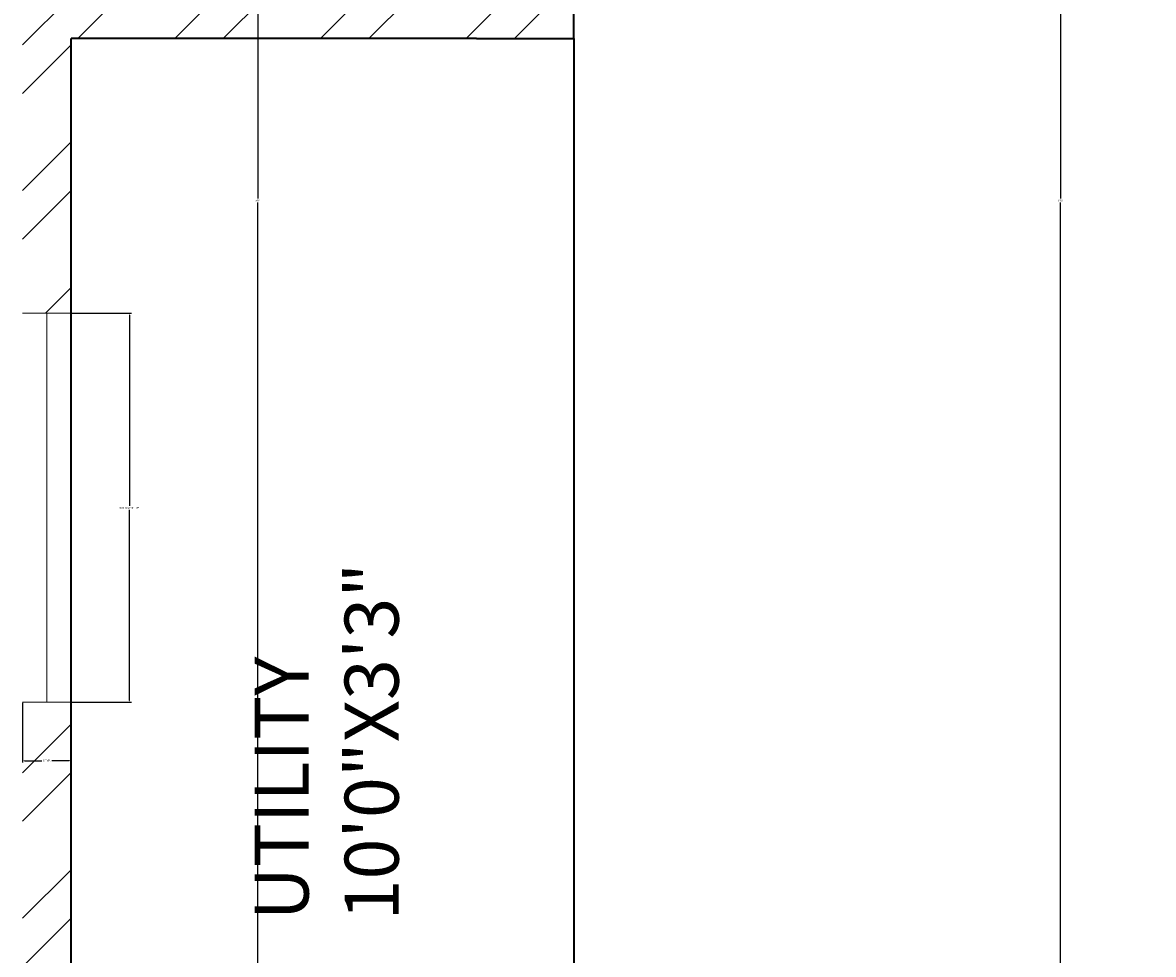
# Model space of a CAD drawing. Units: inches. Extents: x 2120 to 4013, y 1390 to 3019.
# Tile 26 of 59: x 2959 to 3063, y 1878 to 1964. Entities that reach past the tile are written whole.
import ezdxf

# ---------------------------------------------------------------- set-up
doc = ezdxf.new("R2010")
doc.units = ezdxf.units.IN
for name, color, linetype, lineweight in [('A-ANNO-DIMS', 2, 'Continuous', 18), ('A-AREA-IDEN', 7, 'Continuous', 18), ('A-GLAZ', 4, 'Continuous', 18), ('A-WALL', 7, 'Continuous', 35), ('A-WALL-PATT', 252, 'Continuous', 13)]:
    doc.layers.add(name, color=color, linetype=linetype, lineweight=lineweight)
doc.styles.get("Standard").update_dxf_attribs({"font": 'arial.ttf'})
doc.dimstyles.get("Standard").update_dxf_attribs({"dimtxt": 0.18, "dimasz": 0.18, "dimexe": 0.18, "dimexo": 0.0625, "dimgap": 0.09, "dimtad": 0, "dimtih": 1, "dimtoh": 1, "dimdec": 4, "dimzin": 0, "dimdsep": 46, "dimtxsty": 'Standard', "dimcen": 0.09, "dimadec": 0, "dimazin": 0, "dimtfac": 1, "dimtdec": 4, "dimtofl": 0, "dimtmove": 0, "dimatfit": 3, "dimfxl": 1, "dimtolj": 1, "dimtzin": 0, "dimarcsym": 0})

# ---------------------------------------------------------------- blocks, each defined once
blk = doc.blocks.new('WIN-PLAN-36IN-02')
for p, q in [((2.25, 36), (0, 36)), ((0, 36), (4.5, 36)), ((2.25, 0), (2.25, 36)), ((0, 0), (4.5, 0)), ((4.5, 0), (2.25, 0))]:
    blk.add_line(p, q)
blk = doc.blocks.new('*D179')
at = {"layer": 'A-ANNO-DIMS', "color": 0, "lineweight": -2, "transparency": 16777216}
for p, q in [((2963.3, 1937.09), (2968.81, 1937.09)), ((2968.63, 1936.91), (2968.63, 1919.28)), ((2968.63, 1901.27), (2968.63, 1918.91)), ((2963.3, 1901.09), (2968.81, 1901.09))]:
    blk.add_line(p, q, dxfattribs=at)
at = {"layer": 'A-ANNO-DIMS', "color": 0, "transparency": 16777216}
for points in [[(2968.6, 1936.91), (2968.66, 1936.91), (2968.63, 1937.09)], [(2968.6, 1901.27), (2968.66, 1901.27), (2968.63, 1901.09)]]:
    blk.add_solid(points, dxfattribs=at)
at = {"layer": 'Defpoints', "color": 0, "transparency": 16777216}
for p in [(2963.23, 1937.09), (2968.63, 1937.09), (2963.23, 1901.09)]:
    blk.add_point(p, dxfattribs=at)
at = {"layer": 'A-ANNO-DIMS', "color": 0, "transparency": 16777216, "insert": (2968.63, 1919.09), "char_height": 0.18, "attachment_point": 5}
blk.add_mtext('\\A1;WINDOW 36 TYP.', dxfattribs=at)
blk = doc.blocks.new('*D180')
at = {"layer": 'A-ANNO-DIMS', "color": 0, "lineweight": -2, "transparency": 16777216}
for p, q in [((2958.73, 1901.03), (2958.73, 1895.51)), ((2963.23, 1901.03), (2963.23, 1895.51)), ((2958.91, 1895.69), (2960.52, 1895.69)), ((2963.05, 1895.69), (2961.44, 1895.69))]:
    blk.add_line(p, q, dxfattribs=at)
at = {"layer": 'A-ANNO-DIMS', "color": 0, "transparency": 16777216}
for points in [[(2958.91, 1895.72), (2958.91, 1895.66), (2958.73, 1895.69)], [(2963.05, 1895.72), (2963.05, 1895.66), (2963.23, 1895.69)]]:
    blk.add_solid(points, dxfattribs=at)
at = {"layer": 'Defpoints', "color": 0, "transparency": 16777216}
for p in [(2958.73, 1901.09), (2963.23, 1901.09), (2963.23, 1895.69)]:
    blk.add_point(p, dxfattribs=at)
at = {"layer": 'A-ANNO-DIMS', "color": 0, "transparency": 16777216, "insert": (2960.98, 1895.69), "char_height": 0.18, "attachment_point": 5}
blk.add_mtext('\\A1;5 TYP.', dxfattribs=at)
blk = doc.blocks.new('*D212')
at = {"layer": 'A-ANNO-DIMS', "color": 0, "lineweight": -2, "transparency": 16777216}
for p, q in [((3009.8, 2352.53), (3054.91, 2352.53)), ((3054.73, 2352.35), (3054.73, 1947.71)), ((3054.73, 1542.71), (3054.73, 1947.35)), ((3009.8, 1542.53), (3054.91, 1542.53))]:
    blk.add_line(p, q, dxfattribs=at)
at = {"layer": 'A-ANNO-DIMS', "color": 0, "transparency": 16777216}
for points in [[(3054.7, 2352.35), (3054.76, 2352.35), (3054.73, 2352.53)], [(3054.7, 1542.71), (3054.76, 1542.71), (3054.73, 1542.53)]]:
    blk.add_solid(points, dxfattribs=at)
at = {"layer": 'Defpoints', "color": 0, "transparency": 16777216}
for p in [(3009.73, 2352.53), (3009.73, 1542.53), (3054.73, 1542.53)]:
    blk.add_point(p, dxfattribs=at)
at = {"layer": 'A-ANNO-DIMS', "color": 0, "transparency": 16777216, "insert": (3054.73, 1947.53), "char_height": 0.18, "attachment_point": 5}
blk.add_mtext('\\A1;810', dxfattribs=at)
blk = doc.blocks.new('*D217')
at = {"layer": 'A-ANNO-DIMS', "color": 0, "lineweight": -2, "transparency": 16777216}
for p, q in [((3071.67, 2352.53), (2980.31, 2352.53)), ((2980.49, 2352.35), (2980.49, 1947.71)), ((2980.49, 1542.71), (2980.49, 1947.35)), ((3305.67, 1542.53), (2980.31, 1542.53))]:
    blk.add_line(p, q, dxfattribs=at)
at = {"layer": 'A-ANNO-DIMS', "color": 0, "transparency": 16777216}
for points in [[(2980.46, 2352.35), (2980.52, 2352.35), (2980.49, 2352.53)], [(2980.46, 1542.71), (2980.52, 1542.71), (2980.49, 1542.53)]]:
    blk.add_solid(points, dxfattribs=at)
at = {"layer": 'Defpoints', "color": 0, "transparency": 16777216}
for p in [(2980.49, 2352.53), (3071.73, 2352.53), (3305.73, 1542.53)]:
    blk.add_point(p, dxfattribs=at)
at = {"layer": 'A-ANNO-DIMS', "color": 0, "transparency": 16777216, "insert": (2980.49, 1947.53), "char_height": 0.18, "attachment_point": 5}
blk.add_mtext('\\A1;810', dxfattribs=at)

msp = doc.modelspace()

# ---------------------------------------------------------------- hatches: boundary and pattern name
at = {"layer": 'A-WALL-PATT'}
h = msp.add_hatch(dxfattribs=at)
h.set_pattern_fill('ANSI32', color=256)
h.paths.add_polyline_path([(2271.7331, 2343.531), (2283.3788, 2343.531), (2283.3788, 2348.031), (2283.3788, 2352.5306), (2262.7331, 2352.5306), (2262.7331, 2182.638), (2267.2331, 2182.638), (2271.7331, 2182.638), (2271.7331, 2219.031), (2391.7331, 2219.031), (2391.7331, 2214.189), (2393.9831, 2214.189), (2396.2331, 2214.189), (2396.2331, 2219.031), (2420.2331, 2219.031), (2420.2331, 2225.7535), (2417.2197, 2225.7535), (2415.7331, 2225.7535), (2415.7331, 2223.5306), (2271.7331, 2223.5306)])
h.paths.add_polyline_path([(2380.0942, 2352.5306), (2343.3788, 2352.5306), (2343.3788, 2343.531), (2363.2331, 2343.531), (2363.2331, 2288.8489), (2365.4831, 2288.8489), (2367.7331, 2288.8489), (2367.7331, 2343.531), (2380.0942, 2343.531)], flags=17)
h.paths.add_polyline_path([(2432.4339, 2352.5306), (2404.0943, 2352.5306), (2404.0943, 2343.531), (2415.7331, 2343.531), (2415.7331, 2264.0306), (2367.7331, 2264.0306), (2367.7331, 2266.4872), (2363.2331, 2266.4872), (2363.2331, 2259.531), (2367.7331, 2259.531), (2415.7331, 2259.531), (2415.7331, 2255.0658), (2420.2331, 2255.0658), (2420.2331, 2259.531), (2424.5717, 2259.531), (2424.5717, 2261.781), (2424.5717, 2264.0306), (2420.2331, 2264.0306), (2420.2331, 2343.531), (2432.4339, 2343.531)])
h.paths.add_polyline_path([(2508.9115, 2352.5306), (2456.4339, 2352.5306), (2456.4339, 2343.531), (2468.2331, 2343.531), (2468.2331, 2264.0306), (2448.0487, 2264.0306), (2448.0487, 2259.531), (2468.2331, 2259.531), (2468.2331, 2255.5496), (2472.7331, 2255.5496), (2472.7331, 2343.531), (2508.9115, 2343.531)])
h.paths.add_polyline_path([(2637.7331, 2352.5306), (2544.9116, 2352.5306), (2544.9116, 2343.531), (2589.7331, 2343.531), (2633.2331, 2343.531), (2637.7331, 2343.531)])
h.paths.add_polyline_path([(2594.2331, 2343.5306), (2589.7331, 2343.5306), (2589.7331, 2259.5306), (2589.7331, 2252.4915), (2591.9831, 2252.4915), (2594.2331, 2252.4915)])
h.paths.add_polyline_path([(2637.7331, 2223.5306), (2594.2331, 2223.5306), (2594.2331, 2230.1988), (2591.9831, 2230.1988), (2589.7331, 2230.1988), (2589.7331, 2223.5306), (2472.7331, 2223.5306), (2468.2331, 2223.5306), (2468.2331, 2219.031), (2628.7331, 2219.031), (2628.7331, 2138.031), (2637.7331, 2138.031)])
h.paths.add_polyline_path([(3822.6535, 2458.4402), (3874.9468, 2458.4402), (3874.9468, 2476.9866), (3822.6535, 2476.9866)], flags=9)
h.paths.add_polyline_path([(3834.6921, 2781.8174), (3935.9206, 2781.8174), (3935.9206, 2800.3638), (3834.6921, 2800.3638)], flags=9)
h.paths.add_polyline_path([(3832.2843, 2837.9683), (3884.5776, 2837.9683), (3884.5776, 2856.5146), (3832.2843, 2856.5146)], flags=9)
h.paths.add_polyline_path([(3830.9388, 2861.4782), (3956.8958, 2861.4782), (3956.8958, 2880.0245), (3830.9388, 2880.0245)], flags=9)
h.paths.add_polyline_path([(3870.6966, 2352.5752), (3887.9272, 2352.5752), (3887.9272, 2377.3037), (3870.6966, 2377.3037)], flags=9)
h.paths.add_polyline_path([(3289.2701, 2413.161), (3435.2223, 2413.161), (3435.2223, 2450.2538), (3289.2701, 2450.2538)], flags=9)
h.paths.add_polyline_path([(2487.6944, 2414.3601), (2637.8335, 2414.3601), (2637.8335, 2451.4528), (2487.6944, 2451.4528)], flags=9)
h.paths.add_polyline_path([(2567.3724, 1457.9199), (2815.296, 1457.9199), (2815.296, 1495.0127), (2567.3724, 1495.0127)], flags=9)
h.paths.add_polyline_path([(2655.3825, 2093.2363), (2685.9555, 2093.2363), (2685.9555, 2111.8937), (2655.3825, 2111.8937)], flags=9)
h.paths.add_polyline_path([(2543.9218, 1550.6671), (2587.8406, 1550.6671), (2587.8406, 1569.3244), (2543.9218, 1569.3244)], flags=9)
h.paths.add_polyline_path([(2905.1384, 1543.8113), (2949.0572, 1543.8113), (2949.0572, 1562.4686), (2905.1384, 1562.4686)], flags=9)
h.paths.add_polyline_path([(2736.4118, 1702.4736), (2784.2153, 1702.4736), (2784.2153, 1721.1309), (2736.4118, 1721.1309)], flags=9)
h.paths.add_polyline_path([(2912.8666, 1710.4168), (2951.707, 1710.4168), (2951.707, 1729.0741), (2912.8666, 1729.0741)], flags=9)
h.paths.add_polyline_path([(2923.5785, 1763.5038), (2959.7279, 1763.5038), (2959.7279, 1782.1611), (2923.5785, 1782.1611)], flags=9)
h.paths.add_polyline_path([(2925.2114, 1809.6137), (2967.1861, 1809.6137), (2967.1861, 1828.271), (2925.2114, 1828.271)], flags=9)
h.paths.add_polyline_path([(2996.2711, 1878.9003), (2996.2711, 1913.109), (2977.6138, 1913.109), (2977.6138, 1878.9003)], flags=9)
h.paths.add_polyline_path([(2883.0859, 1895.7192), (2927.1855, 1895.7192), (2927.1855, 1914.3766), (2883.0859, 1914.3766)], flags=9)
h.paths.add_polyline_path([(2787.3924, 1810.8013), (2841.0213, 1810.8013), (2841.0213, 1829.4587), (2787.3924, 1829.4587)], flags=9)
h.paths.add_polyline_path([(2775.6399, 2101.7395), (2829.2689, 2101.7395), (2829.2689, 2120.3968), (2775.6399, 2120.3968)], flags=9)
h.paths.add_polyline_path([(2913.0263, 2075.817), (2951.8667, 2075.817), (2951.8667, 2094.4744), (2913.0263, 2094.4744)], flags=9)
h.paths.add_polyline_path([(2929.966, 2133.3669), (2966.1154, 2133.3669), (2966.1154, 2152.0243), (2929.966, 2152.0243)], flags=9)
h.paths.add_polyline_path([(2932.7502, 2182.6088), (2968.8996, 2182.6088), (2968.8996, 2201.2662), (2932.7502, 2201.2662)], flags=9)
h.paths.add_polyline_path([(2996.0681, 2266.3173), (2996.0681, 2300.5261), (2977.4108, 2300.5261), (2977.4108, 2266.3173)], flags=9)
h.paths.add_polyline_path([(2885.1039, 2279.2186), (2929.2035, 2279.2186), (2929.2035, 2297.8759), (2885.1039, 2297.8759)], flags=9)
h.paths.add_polyline_path([(2735.7042, 2218.3197), (2783.5078, 2218.3197), (2783.5078, 2236.9771), (2735.7042, 2236.9771)], flags=9)
h.paths.add_polyline_path([(2635.6049, 2044.0085), (2648.9678, 2044.0085), (2648.9678, 2054.312), (2635.6049, 2054.312)], flags=9)
h.paths.add_polyline_path([(2714.0148, 1923.0473), (2727.3777, 1923.0473), (2727.3777, 1933.3508), (2714.0148, 1933.3508)], flags=9)
h.paths.add_polyline_path([(2709.0345, 1988.1628), (2722.3974, 1988.1628), (2722.3974, 1998.4663), (2709.0345, 1998.4663)], flags=9)
h.paths.add_polyline_path([(2592.8935, 1962.1763), (2606.2564, 1962.1763), (2606.2564, 1972.4799), (2592.8935, 1972.4799)], flags=9)
h.paths.add_polyline_path([(2618.3996, 1985.9724), (2644.1942, 1985.9724), (2644.1942, 1996.2759), (2618.3996, 1996.2759)], flags=9)
h.paths.add_polyline_path([(2601.279, 1920.5869), (2614.6419, 1920.5869), (2614.6419, 1930.8904), (2601.279, 1930.8904)], flags=9)
h.paths.add_polyline_path([(2692.3278, 1932.7645), (2704.5311, 1932.7645), (2704.5311, 1943.0681), (2692.3278, 1943.0681)], flags=9)
h.paths.add_polyline_path([(2311.122, 1672.7318), (2355.0408, 1672.7318), (2355.0408, 1691.3892), (2311.122, 1691.3892)], flags=9)
h.paths.add_polyline_path([(2456.2551, 1632.3198), (2492.4796, 1632.3198), (2492.4796, 1650.9772), (2456.2551, 1650.9772)], flags=9)
h.paths.add_polyline_path([(2401.0766, 1631.4793), (2437.301, 1631.4793), (2437.301, 1650.1367), (2401.0766, 1650.1367)], flags=9)
h.paths.add_polyline_path([(2546.7054, 1700.9235), (2594.509, 1700.9235), (2594.509, 1719.5809), (2546.7054, 1719.5809)], flags=9)
h.paths.add_polyline_path([(2445.4866, 1766.9937), (2497.5261, 1766.9937), (2497.5261, 1785.651), (2445.4866, 1785.651)], flags=9)
h.paths.add_polyline_path([(2287.9992, 1739.7675), (2326.8396, 1739.7675), (2326.8396, 1758.4248), (2287.9992, 1758.4248)], flags=9)
h.paths.add_polyline_path([(2458.5279, 1924.7607), (2510.5675, 1924.7607), (2510.5675, 1943.4181), (2458.5279, 1943.4181)], flags=9)
h.paths.add_polyline_path([(2309.2811, 1902.7642), (2345.4305, 1902.7642), (2345.4305, 1921.4215), (2309.2811, 1921.4215)], flags=9)
h.paths.add_polyline_path([(2490.7554, 2018.9392), (2530.7896, 2018.9392), (2530.7896, 2037.5965), (2490.7554, 2037.5965)], flags=9)
h.paths.add_polyline_path([(2402.143, 2024.7393), (2438.5414, 2024.7393), (2438.5414, 2043.3966), (2402.143, 2043.3966)], flags=9)
h.paths.add_polyline_path([(2287.856, 1931.7926), (2326.6964, 1931.7926), (2326.6964, 1950.4499), (2287.856, 1950.4499)], flags=9)
h.paths.add_polyline_path([(2281.7979, 2193.5771), (2320.6383, 2193.5771), (2320.6383, 2212.2344), (2281.7979, 2212.2344)], flags=25)
h.paths.add_polyline_path([(2484.0754, 2093.892), (2536.115, 2093.892), (2536.115, 2112.5494), (2484.0754, 2112.5494)], flags=9)
h.paths.add_polyline_path([(2624.7948, 2281.8639), (2624.7948, 2311.4137), (2606.1375, 2311.4137), (2606.1375, 2281.8639)], flags=9)
h.paths.add_polyline_path([(2507.5036, 2290.3639), (2541.934, 2290.3639), (2541.934, 2309.0212), (2507.5036, 2309.0212)], flags=9)
h.paths.add_polyline_path([(2423.1076, 2285.2202), (2459.332, 2285.2202), (2459.332, 2303.8776), (2423.1076, 2303.8776)], flags=9)
h.paths.add_polyline_path([(2374.5467, 2289.6272), (2410.7711, 2289.6272), (2410.7711, 2308.2846), (2374.5467, 2308.2846)], flags=25)
h.paths.add_polyline_path([(2277.4907, 2227.5651), (2316.3311, 2227.5651), (2316.3311, 2246.2224), (2277.4907, 2246.2224)], flags=25)
h.paths.add_polyline_path([(2655.3825, 2093.2367), (2685.9555, 2093.2367), (2685.9555, 2111.894), (2655.3825, 2111.894)], flags=9)
h.paths.add_polyline_path([(2543.9217, 1550.6674), (2587.8406, 1550.6674), (2587.8406, 1569.3247), (2543.9217, 1569.3247)], flags=9)
h.paths.add_polyline_path([(2905.1384, 1543.8116), (2949.0572, 1543.8116), (2949.0572, 1562.4689), (2905.1384, 1562.4689)], flags=9)
h.paths.add_polyline_path([(2736.4118, 1702.4739), (2784.2153, 1702.4739), (2784.2153, 1721.1312), (2736.4118, 1721.1312)], flags=9)
h.paths.add_polyline_path([(2912.8666, 1710.4171), (2951.707, 1710.4171), (2951.707, 1729.0744), (2912.8666, 1729.0744)], flags=9)
h.paths.add_polyline_path([(2923.5785, 1763.5041), (2959.7279, 1763.5041), (2959.7279, 1782.1614), (2923.5785, 1782.1614)], flags=9)
h.paths.add_polyline_path([(2925.2114, 1809.614), (2967.1861, 1809.614), (2967.1861, 1828.2713), (2925.2114, 1828.2713)], flags=9)
h.paths.add_polyline_path([(2996.2711, 1878.9006), (2996.2711, 1913.1094), (2977.6137, 1913.1094), (2977.6137, 1878.9006)], flags=9)
h.paths.add_polyline_path([(2883.0859, 1895.7195), (2927.1855, 1895.7195), (2927.1855, 1914.3769), (2883.0859, 1914.3769)], flags=9)
h.paths.add_polyline_path([(2787.3924, 1810.8016), (2841.0213, 1810.8016), (2841.0213, 1829.459), (2787.3924, 1829.459)], flags=9)
h.paths.add_polyline_path([(2775.6399, 2101.7398), (2829.2688, 2101.7398), (2829.2688, 2120.3971), (2775.6399, 2120.3971)], flags=9)
h.paths.add_polyline_path([(2913.0263, 2075.8173), (2951.8667, 2075.8173), (2951.8667, 2094.4747), (2913.0263, 2094.4747)], flags=9)
h.paths.add_polyline_path([(2929.966, 2133.3672), (2966.1154, 2133.3672), (2966.1154, 2152.0246), (2929.966, 2152.0246)], flags=9)
h.paths.add_polyline_path([(2932.7502, 2182.6091), (2968.8996, 2182.6091), (2968.8996, 2201.2665), (2932.7502, 2201.2665)], flags=9)
h.paths.add_polyline_path([(2996.0681, 2266.3176), (2996.0681, 2300.5264), (2977.4108, 2300.5264), (2977.4108, 2266.3176)], flags=9)
h.paths.add_polyline_path([(2885.1039, 2279.2189), (2929.2035, 2279.2189), (2929.2035, 2297.8762), (2885.1039, 2297.8762)], flags=9)
h.paths.add_polyline_path([(2735.7042, 2218.32), (2783.5078, 2218.32), (2783.5078, 2236.9774), (2735.7042, 2236.9774)], flags=9)
h.paths.add_polyline_path([(2635.6048, 2044.0088), (2648.9677, 2044.0088), (2648.9677, 2054.3123), (2635.6048, 2054.3123)], flags=9)
h.paths.add_polyline_path([(2714.0148, 1923.0476), (2727.3777, 1923.0476), (2727.3777, 1933.3511), (2714.0148, 1933.3511)], flags=9)
h.paths.add_polyline_path([(2709.0345, 1988.1631), (2722.3974, 1988.1631), (2722.3974, 1998.4666), (2709.0345, 1998.4666)], flags=9)
h.paths.add_polyline_path([(2592.8935, 1962.1766), (2606.2564, 1962.1766), (2606.2564, 1972.4802), (2592.8935, 1972.4802)], flags=9)
h.paths.add_polyline_path([(2618.3995, 1985.9727), (2644.1942, 1985.9727), (2644.1942, 1996.2762), (2618.3995, 1996.2762)], flags=9)
h.paths.add_polyline_path([(2601.279, 1920.5872), (2614.6419, 1920.5872), (2614.6419, 1930.8908), (2601.279, 1930.8908)], flags=9)
h.paths.add_polyline_path([(2692.3278, 1932.7648), (2704.5311, 1932.7648), (2704.5311, 1943.0684), (2692.3278, 1943.0684)], flags=9)
h.paths.add_polyline_path([(2311.122, 1672.7321), (2355.0408, 1672.7321), (2355.0408, 1691.3895), (2311.122, 1691.3895)], flags=9)
h.paths.add_polyline_path([(2456.2551, 1632.3201), (2492.4795, 1632.3201), (2492.4795, 1650.9775), (2456.2551, 1650.9775)], flags=9)
h.paths.add_polyline_path([(2401.0766, 1631.4796), (2437.301, 1631.4796), (2437.301, 1650.137), (2401.0766, 1650.137)], flags=9)
h.paths.add_polyline_path([(2546.7054, 1700.9238), (2594.509, 1700.9238), (2594.509, 1719.5812), (2546.7054, 1719.5812)], flags=9)
h.paths.add_polyline_path([(2445.4866, 1766.994), (2497.5261, 1766.994), (2497.5261, 1785.6513), (2445.4866, 1785.6513)], flags=9)
h.paths.add_polyline_path([(2287.9992, 1739.7678), (2326.8396, 1739.7678), (2326.8396, 1758.4251), (2287.9992, 1758.4251)], flags=9)
h.paths.add_polyline_path([(2458.5279, 1924.7611), (2510.5675, 1924.7611), (2510.5675, 1943.4184), (2458.5279, 1943.4184)], flags=9)
h.paths.add_polyline_path([(2309.2811, 1902.7645), (2345.4305, 1902.7645), (2345.4305, 1921.4218), (2309.2811, 1921.4218)], flags=9)
h.paths.add_polyline_path([(2490.7554, 2018.9395), (2530.7895, 2018.9395), (2530.7895, 2037.5968), (2490.7554, 2037.5968)], flags=9)
h.paths.add_polyline_path([(2402.143, 2024.7396), (2438.5413, 2024.7396), (2438.5413, 2043.3969), (2402.143, 2043.3969)], flags=9)
h.paths.add_polyline_path([(2287.856, 1931.7929), (2326.6964, 1931.7929), (2326.6964, 1950.4502), (2287.856, 1950.4502)], flags=9)
h.paths.add_polyline_path([(2281.7979, 2193.5774), (2320.6383, 2193.5774), (2320.6383, 2212.2347), (2281.7979, 2212.2347)], flags=25)
h.paths.add_polyline_path([(2484.0754, 2093.8924), (2536.115, 2093.8924), (2536.115, 2112.5497), (2484.0754, 2112.5497)], flags=9)
h.paths.add_polyline_path([(2624.7948, 2281.8642), (2624.7948, 2311.414), (2606.1374, 2311.414), (2606.1374, 2281.8642)], flags=9)
h.paths.add_polyline_path([(2507.5035, 2290.3642), (2541.934, 2290.3642), (2541.934, 2309.0215), (2507.5035, 2309.0215)], flags=9)
h.paths.add_polyline_path([(2423.1075, 2285.2205), (2459.332, 2285.2205), (2459.332, 2303.8779), (2423.1075, 2303.8779)], flags=9)
h.paths.add_polyline_path([(2374.5467, 2289.6275), (2410.7711, 2289.6275), (2410.7711, 2308.2849), (2374.5467, 2308.2849)], flags=25)
h.paths.add_polyline_path([(2277.4907, 2227.5654), (2316.3311, 2227.5654), (2316.3311, 2246.2227), (2277.4907, 2246.2227)], flags=25)
h = msp.add_hatch(dxfattribs=at)
h.set_pattern_fill('ANSI32', color=256)
h.paths.add_polyline_path([(2271.7331, 1980.389), (2262.7331, 1980.389), (2262.7331, 1912.8434), (2267.2331, 1912.8434), (2271.7331, 1912.8434), (2271.7331, 1922.531), (2351.2331, 1922.531), (2351.2331, 1901.4728), (2355.7331, 1901.4728), (2355.7331, 1922.531), (2357.9815, 1922.531), (2357.9815, 1926.5306), (2271.7331, 1926.5306)])
h.paths.add_polyline_path([(2589.2331, 1949.1622), (2584.7331, 1949.1622), (2580.2331, 1949.1622), (2580.2331, 1874.5306), (2355.7331, 1874.5306), (2355.7331, 1880.1922), (2351.2331, 1880.1922), (2351.2331, 1874.5306), (2271.7331, 1874.5306), (2271.7331, 1888.8431), (2262.7331, 1888.8431), (2262.7331, 1842.2909), (2267.2331, 1842.2909), (2271.7331, 1842.2909), (2271.7331, 1865.531), (2415.7331, 1865.531), (2415.7331, 1779.7286), (2420.2331, 1779.7286), (2420.2331, 1865.531), (2589.2331, 1865.531)])
h.paths.add_polyline_path([(2271.7331, 1782.2906), (2262.7331, 1782.2906), (2262.7331, 1711.4639), (2267.2331, 1711.4639), (2271.7331, 1711.4639), (2271.7331, 1738.031), (2420.2331, 1738.031), (2420.2331, 1742.531), (2420.2331, 1747.3376), (2417.9831, 1747.3376), (2415.7331, 1747.3376), (2415.7331, 1742.5306), (2271.7331, 1742.5306)])
h.paths.add_polyline_path([(2271.7331, 1627.031), (2362.3957, 1627.031), (2362.3957, 1629.281), (2362.3957, 1631.5306), (2271.7331, 1631.5306), (2271.7331, 1675.4636), (2262.7331, 1675.4636), (2262.7331, 1581.531), (2405.3032, 1581.531), (2405.3032, 1586.031), (2405.3032, 1590.5306), (2396.2331, 1590.5306), (2396.2331, 1691.4513), (2418.7206, 1691.4513), (2418.7206, 1695.951), (2396.2331, 1695.951), (2391.7331, 1695.951), (2391.7331, 1631.5306), (2386.7425, 1631.5306), (2386.7425, 1629.2806), (2386.7425, 1627.031), (2391.7331, 1627.031), (2391.7331, 1586.1709), (2271.7331, 1586.1709)])
h.paths.add_polyline_path([(2459.6703, 1590.5306), (2429.3032, 1590.5306), (2429.3032, 1581.531), (2459.6703, 1581.531), (2459.6703, 1586.031)])
h.paths.add_polyline_path([(2501.2331, 1590.531), (2501.2331, 1665.0195), (2498.9831, 1665.0195), (2496.7331, 1665.0195), (2496.7331, 1590.5306), (2483.8201, 1590.5306), (2483.8201, 1590.1579), (2483.6704, 1590.1579), (2483.6704, 1581.531), (2505.0196, 1581.531), (2505.0196, 1583.781), (2505.0196, 1586.0306), (2501.2331, 1586.0306)])
h.paths.add_polyline_path([(2544.1361, 1583.781), (2544.1361, 1586.0306), (2527.1368, 1586.0306), (2527.1368, 1583.7806), (2527.1368, 1581.531), (2544.1361, 1581.531)])
h.paths.add_polyline_path([(3822.6535, 2458.4402), (3874.9468, 2458.4402), (3874.9468, 2476.9866), (3822.6535, 2476.9866)], flags=9)
h.paths.add_polyline_path([(3834.6921, 2781.8174), (3935.9206, 2781.8174), (3935.9206, 2800.3638), (3834.6921, 2800.3638)], flags=9)
h.paths.add_polyline_path([(3832.2843, 2837.9683), (3884.5776, 2837.9683), (3884.5776, 2856.5146), (3832.2843, 2856.5146)], flags=9)
h.paths.add_polyline_path([(3830.9388, 2861.4782), (3956.8958, 2861.4782), (3956.8958, 2880.0245), (3830.9388, 2880.0245)], flags=9)
h.paths.add_polyline_path([(3870.6966, 2352.5752), (3887.9272, 2352.5752), (3887.9272, 2377.3037), (3870.6966, 2377.3037)], flags=9)
h.paths.add_polyline_path([(3289.2701, 2413.161), (3435.2223, 2413.161), (3435.2223, 2450.2538), (3289.2701, 2450.2538)], flags=9)
h.paths.add_polyline_path([(2487.6944, 2414.3601), (2637.8335, 2414.3601), (2637.8335, 2451.4528), (2487.6944, 2451.4528)], flags=9)
h.paths.add_polyline_path([(2567.3724, 1457.9199), (2815.296, 1457.9199), (2815.296, 1495.0127), (2567.3724, 1495.0127)], flags=9)
h.paths.add_polyline_path([(2655.3825, 2093.2363), (2685.9555, 2093.2363), (2685.9555, 2111.8937), (2655.3825, 2111.8937)], flags=9)
h.paths.add_polyline_path([(2543.9218, 1550.6671), (2587.8406, 1550.6671), (2587.8406, 1569.3244), (2543.9218, 1569.3244)], flags=9)
h.paths.add_polyline_path([(2905.1384, 1543.8113), (2949.0572, 1543.8113), (2949.0572, 1562.4686), (2905.1384, 1562.4686)], flags=9)
h.paths.add_polyline_path([(2736.4118, 1702.4736), (2784.2153, 1702.4736), (2784.2153, 1721.1309), (2736.4118, 1721.1309)], flags=9)
h.paths.add_polyline_path([(2912.8666, 1710.4168), (2951.707, 1710.4168), (2951.707, 1729.0741), (2912.8666, 1729.0741)], flags=9)
h.paths.add_polyline_path([(2923.5785, 1763.5038), (2959.7279, 1763.5038), (2959.7279, 1782.1611), (2923.5785, 1782.1611)], flags=9)
h.paths.add_polyline_path([(2925.2114, 1809.6137), (2967.1861, 1809.6137), (2967.1861, 1828.271), (2925.2114, 1828.271)], flags=9)
h.paths.add_polyline_path([(2996.2711, 1878.9003), (2996.2711, 1913.109), (2977.6138, 1913.109), (2977.6138, 1878.9003)], flags=9)
h.paths.add_polyline_path([(2883.0859, 1895.7192), (2927.1855, 1895.7192), (2927.1855, 1914.3766), (2883.0859, 1914.3766)], flags=9)
h.paths.add_polyline_path([(2787.3924, 1810.8013), (2841.0213, 1810.8013), (2841.0213, 1829.4587), (2787.3924, 1829.4587)], flags=9)
h.paths.add_polyline_path([(2775.6399, 2101.7395), (2829.2689, 2101.7395), (2829.2689, 2120.3968), (2775.6399, 2120.3968)], flags=9)
h.paths.add_polyline_path([(2913.0263, 2075.817), (2951.8667, 2075.817), (2951.8667, 2094.4744), (2913.0263, 2094.4744)], flags=9)
h.paths.add_polyline_path([(2929.966, 2133.3669), (2966.1154, 2133.3669), (2966.1154, 2152.0243), (2929.966, 2152.0243)], flags=9)
h.paths.add_polyline_path([(2932.7502, 2182.6088), (2968.8996, 2182.6088), (2968.8996, 2201.2662), (2932.7502, 2201.2662)], flags=9)
h.paths.add_polyline_path([(2996.0681, 2266.3173), (2996.0681, 2300.5261), (2977.4108, 2300.5261), (2977.4108, 2266.3173)], flags=9)
h.paths.add_polyline_path([(2885.1039, 2279.2186), (2929.2035, 2279.2186), (2929.2035, 2297.8759), (2885.1039, 2297.8759)], flags=9)
h.paths.add_polyline_path([(2735.7042, 2218.3197), (2783.5078, 2218.3197), (2783.5078, 2236.9771), (2735.7042, 2236.9771)], flags=9)
h.paths.add_polyline_path([(2635.6049, 2044.0085), (2648.9678, 2044.0085), (2648.9678, 2054.312), (2635.6049, 2054.312)], flags=9)
h.paths.add_polyline_path([(2714.0148, 1923.0473), (2727.3777, 1923.0473), (2727.3777, 1933.3508), (2714.0148, 1933.3508)], flags=9)
h.paths.add_polyline_path([(2709.0345, 1988.1628), (2722.3974, 1988.1628), (2722.3974, 1998.4663), (2709.0345, 1998.4663)], flags=9)
h.paths.add_polyline_path([(2592.8935, 1962.1763), (2606.2564, 1962.1763), (2606.2564, 1972.4799), (2592.8935, 1972.4799)], flags=9)
h.paths.add_polyline_path([(2618.3996, 1985.9724), (2644.1942, 1985.9724), (2644.1942, 1996.2759), (2618.3996, 1996.2759)], flags=9)
h.paths.add_polyline_path([(2601.279, 1920.5869), (2614.6419, 1920.5869), (2614.6419, 1930.8904), (2601.279, 1930.8904)], flags=9)
h.paths.add_polyline_path([(2692.3278, 1932.7645), (2704.5311, 1932.7645), (2704.5311, 1943.0681), (2692.3278, 1943.0681)], flags=9)
h.paths.add_polyline_path([(2311.122, 1672.7318), (2355.0408, 1672.7318), (2355.0408, 1691.3892), (2311.122, 1691.3892)], flags=25)
h.paths.add_polyline_path([(2456.2551, 1632.3198), (2492.4796, 1632.3198), (2492.4796, 1650.9772), (2456.2551, 1650.9772)], flags=9)
h.paths.add_polyline_path([(2401.0766, 1631.4793), (2437.301, 1631.4793), (2437.301, 1650.1367), (2401.0766, 1650.1367)], flags=9)
h.paths.add_polyline_path([(2546.7054, 1700.9235), (2594.509, 1700.9235), (2594.509, 1719.5809), (2546.7054, 1719.5809)], flags=9)
h.paths.add_polyline_path([(2445.4866, 1766.9937), (2497.5261, 1766.9937), (2497.5261, 1785.651), (2445.4866, 1785.651)], flags=9)
h.paths.add_polyline_path([(2287.9992, 1739.7675), (2326.8396, 1739.7675), (2326.8396, 1758.4248), (2287.9992, 1758.4248)], flags=24)
h.paths.add_polyline_path([(2458.5279, 1924.7607), (2510.5675, 1924.7607), (2510.5675, 1943.4181), (2458.5279, 1943.4181)], flags=25)
h.paths.add_polyline_path([(2309.2811, 1902.7642), (2345.4305, 1902.7642), (2345.4305, 1921.4215), (2309.2811, 1921.4215)], flags=25)
h.paths.add_polyline_path([(2490.7554, 2018.9392), (2530.7896, 2018.9392), (2530.7896, 2037.5965), (2490.7554, 2037.5965)], flags=9)
h.paths.add_polyline_path([(2402.143, 2024.7393), (2438.5414, 2024.7393), (2438.5414, 2043.3966), (2402.143, 2043.3966)], flags=9)
h.paths.add_polyline_path([(2287.856, 1931.7926), (2326.6964, 1931.7926), (2326.6964, 1950.4499), (2287.856, 1950.4499)], flags=25)
h.paths.add_polyline_path([(2281.7979, 2193.5771), (2320.6383, 2193.5771), (2320.6383, 2212.2344), (2281.7979, 2212.2344)], flags=9)
h.paths.add_polyline_path([(2484.0754, 2093.892), (2536.115, 2093.892), (2536.115, 2112.5494), (2484.0754, 2112.5494)], flags=9)
h.paths.add_polyline_path([(2624.7948, 2281.8639), (2624.7948, 2311.4137), (2606.1375, 2311.4137), (2606.1375, 2281.8639)], flags=9)
h.paths.add_polyline_path([(2507.5036, 2290.3639), (2541.934, 2290.3639), (2541.934, 2309.0212), (2507.5036, 2309.0212)], flags=9)
h.paths.add_polyline_path([(2423.1076, 2285.2202), (2459.332, 2285.2202), (2459.332, 2303.8776), (2423.1076, 2303.8776)], flags=9)
h.paths.add_polyline_path([(2374.5467, 2289.6272), (2410.7711, 2289.6272), (2410.7711, 2308.2846), (2374.5467, 2308.2846)], flags=9)
h.paths.add_polyline_path([(2277.4907, 2227.5651), (2316.3311, 2227.5651), (2316.3311, 2246.2224), (2277.4907, 2246.2224)], flags=9)
h.paths.add_polyline_path([(2655.3825, 2093.2367), (2685.9555, 2093.2367), (2685.9555, 2111.894), (2655.3825, 2111.894)], flags=9)
h.paths.add_polyline_path([(2543.9217, 1550.6674), (2587.8406, 1550.6674), (2587.8406, 1569.3247), (2543.9217, 1569.3247)], flags=9)
h.paths.add_polyline_path([(2905.1384, 1543.8116), (2949.0572, 1543.8116), (2949.0572, 1562.4689), (2905.1384, 1562.4689)], flags=9)
h.paths.add_polyline_path([(2736.4118, 1702.4739), (2784.2153, 1702.4739), (2784.2153, 1721.1312), (2736.4118, 1721.1312)], flags=9)
h.paths.add_polyline_path([(2912.8666, 1710.4171), (2951.707, 1710.4171), (2951.707, 1729.0744), (2912.8666, 1729.0744)], flags=9)
h.paths.add_polyline_path([(2923.5785, 1763.5041), (2959.7279, 1763.5041), (2959.7279, 1782.1614), (2923.5785, 1782.1614)], flags=9)
h.paths.add_polyline_path([(2925.2114, 1809.614), (2967.1861, 1809.614), (2967.1861, 1828.2713), (2925.2114, 1828.2713)], flags=9)
h.paths.add_polyline_path([(2996.2711, 1878.9006), (2996.2711, 1913.1094), (2977.6137, 1913.1094), (2977.6137, 1878.9006)], flags=9)
h.paths.add_polyline_path([(2883.0859, 1895.7195), (2927.1855, 1895.7195), (2927.1855, 1914.3769), (2883.0859, 1914.3769)], flags=9)
h.paths.add_polyline_path([(2787.3924, 1810.8016), (2841.0213, 1810.8016), (2841.0213, 1829.459), (2787.3924, 1829.459)], flags=9)
h.paths.add_polyline_path([(2775.6399, 2101.7398), (2829.2688, 2101.7398), (2829.2688, 2120.3971), (2775.6399, 2120.3971)], flags=9)
h.paths.add_polyline_path([(2913.0263, 2075.8173), (2951.8667, 2075.8173), (2951.8667, 2094.4747), (2913.0263, 2094.4747)], flags=9)
h.paths.add_polyline_path([(2929.966, 2133.3672), (2966.1154, 2133.3672), (2966.1154, 2152.0246), (2929.966, 2152.0246)], flags=9)
h.paths.add_polyline_path([(2932.7502, 2182.6091), (2968.8996, 2182.6091), (2968.8996, 2201.2665), (2932.7502, 2201.2665)], flags=9)
h.paths.add_polyline_path([(2996.0681, 2266.3176), (2996.0681, 2300.5264), (2977.4108, 2300.5264), (2977.4108, 2266.3176)], flags=9)
h.paths.add_polyline_path([(2885.1039, 2279.2189), (2929.2035, 2279.2189), (2929.2035, 2297.8762), (2885.1039, 2297.8762)], flags=9)
h.paths.add_polyline_path([(2735.7042, 2218.32), (2783.5078, 2218.32), (2783.5078, 2236.9774), (2735.7042, 2236.9774)], flags=9)
h.paths.add_polyline_path([(2635.6048, 2044.0088), (2648.9677, 2044.0088), (2648.9677, 2054.3123), (2635.6048, 2054.3123)], flags=9)
h.paths.add_polyline_path([(2714.0148, 1923.0476), (2727.3777, 1923.0476), (2727.3777, 1933.3511), (2714.0148, 1933.3511)], flags=9)
h.paths.add_polyline_path([(2709.0345, 1988.1631), (2722.3974, 1988.1631), (2722.3974, 1998.4666), (2709.0345, 1998.4666)], flags=9)
h.paths.add_polyline_path([(2592.8935, 1962.1766), (2606.2564, 1962.1766), (2606.2564, 1972.4802), (2592.8935, 1972.4802)], flags=9)
h.paths.add_polyline_path([(2618.3995, 1985.9727), (2644.1942, 1985.9727), (2644.1942, 1996.2762), (2618.3995, 1996.2762)], flags=9)
h.paths.add_polyline_path([(2601.279, 1920.5872), (2614.6419, 1920.5872), (2614.6419, 1930.8908), (2601.279, 1930.8908)], flags=9)
h.paths.add_polyline_path([(2692.3278, 1932.7648), (2704.5311, 1932.7648), (2704.5311, 1943.0684), (2692.3278, 1943.0684)], flags=9)
h.paths.add_polyline_path([(2311.122, 1672.7321), (2355.0408, 1672.7321), (2355.0408, 1691.3895), (2311.122, 1691.3895)], flags=25)
h.paths.add_polyline_path([(2456.2551, 1632.3201), (2492.4795, 1632.3201), (2492.4795, 1650.9775), (2456.2551, 1650.9775)], flags=9)
h.paths.add_polyline_path([(2401.0766, 1631.4796), (2437.301, 1631.4796), (2437.301, 1650.137), (2401.0766, 1650.137)], flags=9)
h.paths.add_polyline_path([(2546.7054, 1700.9238), (2594.509, 1700.9238), (2594.509, 1719.5812), (2546.7054, 1719.5812)], flags=9)
h.paths.add_polyline_path([(2445.4866, 1766.994), (2497.5261, 1766.994), (2497.5261, 1785.6513), (2445.4866, 1785.6513)], flags=9)
h.paths.add_polyline_path([(2287.9992, 1739.7678), (2326.8396, 1739.7678), (2326.8396, 1758.4251), (2287.9992, 1758.4251)], flags=24)
h.paths.add_polyline_path([(2458.5279, 1924.7611), (2510.5675, 1924.7611), (2510.5675, 1943.4184), (2458.5279, 1943.4184)], flags=25)
h.paths.add_polyline_path([(2309.2811, 1902.7645), (2345.4305, 1902.7645), (2345.4305, 1921.4218), (2309.2811, 1921.4218)], flags=25)
h.paths.add_polyline_path([(2490.7554, 2018.9395), (2530.7895, 2018.9395), (2530.7895, 2037.5968), (2490.7554, 2037.5968)], flags=9)
h.paths.add_polyline_path([(2402.143, 2024.7396), (2438.5413, 2024.7396), (2438.5413, 2043.3969), (2402.143, 2043.3969)], flags=9)
h.paths.add_polyline_path([(2287.856, 1931.7929), (2326.6964, 1931.7929), (2326.6964, 1950.4502), (2287.856, 1950.4502)], flags=25)
h.paths.add_polyline_path([(2281.7979, 2193.5774), (2320.6383, 2193.5774), (2320.6383, 2212.2347), (2281.7979, 2212.2347)], flags=9)
h.paths.add_polyline_path([(2484.0754, 2093.8924), (2536.115, 2093.8924), (2536.115, 2112.5497), (2484.0754, 2112.5497)], flags=9)
h.paths.add_polyline_path([(2624.7948, 2281.8642), (2624.7948, 2311.414), (2606.1374, 2311.414), (2606.1374, 2281.8642)], flags=9)
h.paths.add_polyline_path([(2507.5035, 2290.3642), (2541.934, 2290.3642), (2541.934, 2309.0215), (2507.5035, 2309.0215)], flags=9)
h.paths.add_polyline_path([(2423.1075, 2285.2205), (2459.332, 2285.2205), (2459.332, 2303.8779), (2423.1075, 2303.8779)], flags=9)
h.paths.add_polyline_path([(2374.5467, 2289.6275), (2410.7711, 2289.6275), (2410.7711, 2308.2849), (2374.5467, 2308.2849)], flags=9)
h.paths.add_polyline_path([(2277.4907, 2227.5654), (2316.3311, 2227.5654), (2316.3311, 2246.2227), (2277.4907, 2246.2227)], flags=9)
h = msp.add_hatch(dxfattribs=at)
h.set_pattern_fill('ANSI32', color=256)
h.paths.add_polyline_path([(2271.7331, 2122.6377), (2262.7331, 2122.6377), (2262.7331, 2040.3893), (2267.2331, 2040.3893), (2271.7331, 2040.3893), (2271.7331, 2044.8856), (2271.7331, 2070.531), (2391.7331, 2070.531), (2391.7331, 1926.5306), (2388.3993, 1926.5306), (2388.3993, 1922.531), (2395.7331, 1922.531), (2395.7331, 1992.531), (2400.4511, 1992.531), (2400.4511, 1997.0306), (2395.7331, 1997.0306), (2395.7331, 2070.531), (2443.7331, 2070.531), (2443.7331, 2046.1368), (2448.2331, 2046.1368), (2448.2331, 2070.531), (2580.2331, 2070.531), (2580.2331, 1997.0306), (2492.9076, 1997.0306), (2492.9076, 1992.531), (2580.2331, 1992.531), (2580.2331, 1983.9368), (2589.2331, 1983.9368), (2589.2331, 2070.531), (2589.2331, 2075.0306), (2396.2331, 2075.0306), (2396.2331, 2184.3565), (2393.9831, 2184.3565), (2391.7331, 2184.3565), (2391.7331, 2075.0306), (2271.7331, 2075.0306)])
h.paths.add_polyline_path([(2724.7331, 2138.0306), (2628.7331, 2138.0306), (2628.7331, 2070.5306), (2628.7331, 2067.0987), (2633.2331, 2067.0987), (2637.7331, 2067.0987), (2637.7331, 2070.531), (2657.3413, 2070.531), (2657.3413, 2079.5306), (2637.7331, 2079.5306), (2637.7331, 2129.031), (2715.7331, 2129.031), (2715.7331, 2079.5306), (2698.0378, 2079.5306), (2698.0378, 2070.531), (2715.7331, 2070.531), (2715.7331, 2012.1531), (2720.2331, 2012.1531), (2724.7331, 2012.1531)])
h.paths.add_polyline_path([(2724.7331, 2213.031), (2831.3209, 2213.031), (2831.3209, 2215.281), (2831.3209, 2217.5306), (2724.7331, 2217.5306), (2724.7331, 2343.531), (2751.8755, 2343.531), (2751.8755, 2352.5306), (2715.7331, 2352.5306), (2715.7331, 2138.031), (2724.7331, 2138.031)])
h.paths.add_polyline_path([(2902.53, 2352.5306), (2811.8755, 2352.5306), (2811.8755, 2343.531), (2867.2331, 2343.531), (2867.2331, 2217.5306), (2863.6364, 2217.5306), (2863.6364, 2213.031), (2871.7331, 2213.031), (2871.7331, 2217.531), (2871.7331, 2343.531), (2902.53, 2343.531)])
h.paths.add_polyline_path([(3009.7331, 2352.5306), (2938.53, 2352.5306), (2938.53, 2343.531), (2966.2331, 2343.531), (2966.2331, 2242.3281), (2968.4831, 2242.3281), (2970.7331, 2242.3281), (2970.7331, 2343.531), (3009.7331, 2343.531)])
h.paths.add_polyline_path([(3009.7331, 2217.5306), (2970.7331, 2217.5306), (2970.7331, 2220.5422), (2968.4831, 2220.5422), (2966.2331, 2220.5422), (2966.2331, 2217.5306), (2911.7752, 2217.5306), (2907.7331, 2217.5306), (2907.7331, 2213.0306), (2907.7331, 2194.9663), (2912.2331, 2194.9663), (2912.2331, 2213.031), (2970.7331, 2213.031), (3000.7331, 2213.031), (3000.7331, 2205.523), (3009.7331, 2205.523)])
h.paths.add_polyline_path([(3009.7331, 2181.5227), (3000.7331, 2181.5227), (3000.7331, 2165.0306), (2912.2331, 2165.0306), (2912.2331, 2170.8202), (2907.7331, 2170.8202), (2907.7331, 2165.0306), (2899.5169, 2165.0306), (2899.5169, 2162.7806), (2899.5169, 2160.531), (2907.7331, 2160.531), (2907.7331, 2137.3432), (2912.2331, 2137.3432), (2912.2331, 2160.531), (3000.7331, 2160.531), (3000.7331, 2150.4993), (3009.7331, 2150.4993)])
h.paths.add_polyline_path([(3009.7331, 2126.499), (3005.2331, 2126.499), (3000.7331, 2126.499), (3000.7331, 2112.5306), (2912.2331, 2112.5306), (2912.2331, 2115.6036), (2907.7331, 2115.6036), (2907.7331, 2108.031), (3000.7331, 2108.031), (3000.7331, 2084.7256), (3009.7331, 2084.7256)], flags=17)
h.paths.add_polyline_path([(3009.7331, 1971.531), (3009.7331, 2024.7253), (3000.7331, 2024.7253), (3000.7331, 2006.4153), (3000.7331, 1971.5306), (2864.2331, 1971.5306), (2864.2331, 2160.531), (2868.0522, 2160.531), (2868.0522, 2165.0306), (2859.7331, 2165.0306), (2859.7331, 1971.5306), (2724.7331, 1971.5306), (2724.7331, 1977.7012), (2715.7331, 1977.7012), (2715.7331, 1962.5306), (2715.7331, 1950.9035), (2720.2331, 1950.9035), (2724.7331, 1950.9035), (2724.7331, 1962.531), (2855.2331, 1962.531), (2859.7331, 1962.531), (2859.7331, 1835.031), (2864.2331, 1834.8158), (2864.2331, 1962.531), (2958.7331, 1962.531), (2958.7331, 1937.0925), (2963.2331, 1937.0925), (2963.2331, 1962.531), (3000.7331, 1962.531), (3009.7331, 1962.531)])
h.paths.add_polyline_path([(2724.7331, 1728.531), (2822.7164, 1728.531), (2822.7164, 1733.0306), (2724.7331, 1733.0306), (2724.7331, 1779.3416), (2715.7331, 1779.3416), (2715.7331, 1581.531), (2753.02, 1581.531), (2753.02, 1586.031), (2753.02, 1590.5306), (2724.7331, 1590.5306)])
h.paths.add_polyline_path([(2864.2331, 1590.531), (2864.2331, 1787.031), (2868.4075, 1787.031), (2868.4075, 1791.5306), (2859.7331, 1791.5306), (2859.7331, 1739.0306), (2859.7331, 1733.0306), (2854.3125, 1733.0306), (2854.3125, 1728.531), (2859.7331, 1728.531), (2859.7331, 1590.5306), (2813.02, 1590.5306), (2813.02, 1581.531), (2868.4123, 1581.531), (2868.4123, 1583.781), (2868.4123, 1586.0306), (2864.2331, 1586.0306)])
h.paths.add_polyline_path([(3009.7331, 1754.6619), (3000.7331, 1754.6619), (3000.7331, 1739.0306), (2912.2331, 1739.0306), (2912.2331, 1742.2257), (2907.7331, 1742.2257), (2907.7331, 1739.0306), (2907.7331, 1734.531), (3000.7331, 1734.531), (3000.7331, 1590.5306), (3000.7331, 1586.0306), (2971.3921, 1586.0306), (2971.3921, 1581.531), (3009.7331, 1581.531)])
h.paths.add_polyline_path([(2911.3921, 1583.781), (2911.3921, 1586.0306), (2891.2138, 1586.0306), (2891.2138, 1581.531), (2911.3921, 1581.531)])
h.paths.add_polyline_path([(3009.7331, 1799.8422), (3000.7331, 1799.8422), (3000.7331, 1791.5306), (2912.2331, 1791.5306), (2912.2331, 1796.3264), (2909.9831, 1796.3264), (2907.7331, 1796.3264), (2907.7331, 1791.5306), (2902.7033, 1791.5306), (2902.7033, 1787.031), (2907.7331, 1787.031), (2907.7331, 1761.1622), (2912.2331, 1761.1622), (2912.2331, 1787.031), (3000.7331, 1787.031), (3000.7331, 1778.6622), (3009.7331, 1778.6622)])
h.paths.add_polyline_path([(3009.7331, 1839.5306), (2963.2331, 1839.5306), (2963.2331, 1842.8629), (2960.9831, 1842.8629), (2958.7331, 1842.8629), (2958.7331, 1839.5306), (2907.7331, 1839.5306), (2907.7331, 1814.4599), (2912.2331, 1814.4599), (2912.2331, 1835.031), (3000.7331, 1835.031), (3000.7331, 1823.8425), (3009.7331, 1823.8425), (3009.7331, 1835.031)])
h.paths.add_polyline_path([(2963.2331, 1901.0922), (2960.9831, 1901.0922), (2958.7331, 1901.0922), (2958.7331, 1862.8843), (2963.2331, 1862.8843)], flags=17)
h.paths.add_polyline_path([(2724.7331, 1891.9826), (2724.7331, 1914.3416), (2715.7331, 1914.3416), (2715.7331, 1783.8416), (2637.7331, 1783.8416), (2637.7331, 1914.3416), (2628.7331, 1914.3416), (2624.7701, 1914.3416), (2624.7701, 1909.8416), (2624.7701, 1905.3419), (2628.7331, 1905.3419), (2628.7331, 1876.9915), (2628.7331, 1779.3419), (2637.7331, 1779.3419), (2715.7331, 1779.3419), (2724.7331, 1779.3419), (2724.7331, 1835.031)])
h.paths.add_polyline_path([(2637.7331, 1731.531), (2637.7331, 1779.3416), (2628.7331, 1779.3416), (2628.7331, 1731.5306), (2589.2331, 1731.5306), (2535.9814, 1731.5306), (2496.7331, 1731.5306), (2496.7331, 1725.6876), (2498.9831, 1725.6876), (2501.2331, 1725.6876), (2501.2331, 1727.031), (2628.7331, 1727.031), (2628.7331, 1680.4203), (2628.7331, 1590.5306), (2628.7331, 1586.0306), (2604.1361, 1586.0306), (2604.1361, 1581.531), (2637.7331, 1581.531), (2637.7331, 1590.531)])

# ---------------------------------------------------------------- linework, layer by layer
at = {"layer": 'A-WALL'}
for p, q in [((3009.7331, 1962.531), (3009.7331, 1971.531)), ((3009.7331, 1962.5306), (3009.7331, 1971.5306)), ((3000.7331, 1962.531), (2963.2331, 1962.531)), ((2963.2331, 1861.6427), (2963.2331, 1962.531)), ((2963.2331, 1861.6424), (2963.2331, 1962.5306)), ((3000.7331, 1962.5306), (2963.2331, 1962.5306)), ((3000.7331, 1962.531), (3009.7331, 1962.531)), ((3000.7331, 1962.5306), (3009.7331, 1962.5306)), ((3009.7331, 1962.531), (3009.7331, 1542.531)), ((3009.7331, 1962.5306), (3009.7331, 1542.5306))]:
    msp.add_line(p, q, dxfattribs=at)

# ---------------------------------------------------------------- block references
at = {"layer": 'A-GLAZ'}
for p in [(2958.7331, 1901.0925), (2958.7331, 1901.0922)]:
    msp.add_blockref('WIN-PLAN-36IN-02', p, dxfattribs=at)

# ---------------------------------------------------------------- texts
at = {"layer": 'A-AREA-IDEN', "char_height": 5, "attachment_point": 1, "rotation": 90}
for insert in [(2980.1871, 1880.9112), (2980.1871, 1880.9109)]:
    msp.add_mtext_dynamic_manual_height_columns('UTILITY\\P10\'0"X3\'3"', width=204.664663, gutter_width=12.5, heights=[0], dxfattribs=dict(at, insert=insert))

# ---------------------------------------------------------------- dimensions: what is measured, and where the dimension line sits
at = {"layer": 'A-ANNO-DIMS'}
for base, p1, p2, picture, middle in [((2980.4877, 2352.531), (3305.7347, 1542.531), (3071.7347, 2352.531), '*D217', (2980.4877, 1947.531)), ((3054.7331, 1542.531), (3009.7331, 2352.531), (3009.7331, 1542.531), '*D212', (3054.7331, 1947.531))]:
    dim = msp.add_linear_dim(base=base, p1=p1, p2=p2, angle=90, dimstyle='Standard', override={"dimdec": 0, "dimlfac": 1, "dimrnd": 0, "dimzin": 0, "dimdsep": 46, "dimlunit": 2}, dxfattribs=at)
    dim.commit()
    dim.dimension.update_dxf_attribs({"geometry": picture, "text_midpoint": middle})
dim = msp.add_linear_dim(base=(2968.6331, 1937.0925), p1=(2963.2331, 1901.0925), p2=(2963.2331, 1937.0925), angle=90, text='WINDOW <> TYP.', dimstyle='Standard', override={"dimdec": 0, "dimlfac": 1, "dimrnd": 0, "dimzin": 0, "dimdsep": 46, "dimlunit": 2}, dxfattribs=at)
dim.commit()
dim.dimension.update_dxf_attribs({"geometry": '*D179', "text_midpoint": (2968.6331, 1919.0925)})
dim = msp.add_linear_dim(base=(2963.2331222497, 1895.6925467185), p1=(2958.7331222497, 1901.0925467185), p2=(2963.2331222497, 1901.0925467185), text='<> TYP.', dimstyle='Standard', override={"dimdec": 0, "dimlfac": 1, "dimrnd": 0, "dimzin": 0, "dimdsep": 46, "dimlunit": 2}, dxfattribs=at)
dim.commit()
dim.dimension.update_dxf_attribs({"geometry": '*D180', "text_midpoint": (2960.9831222497, 1895.6925467185)})

doc.saveas('drawing.dxf')
